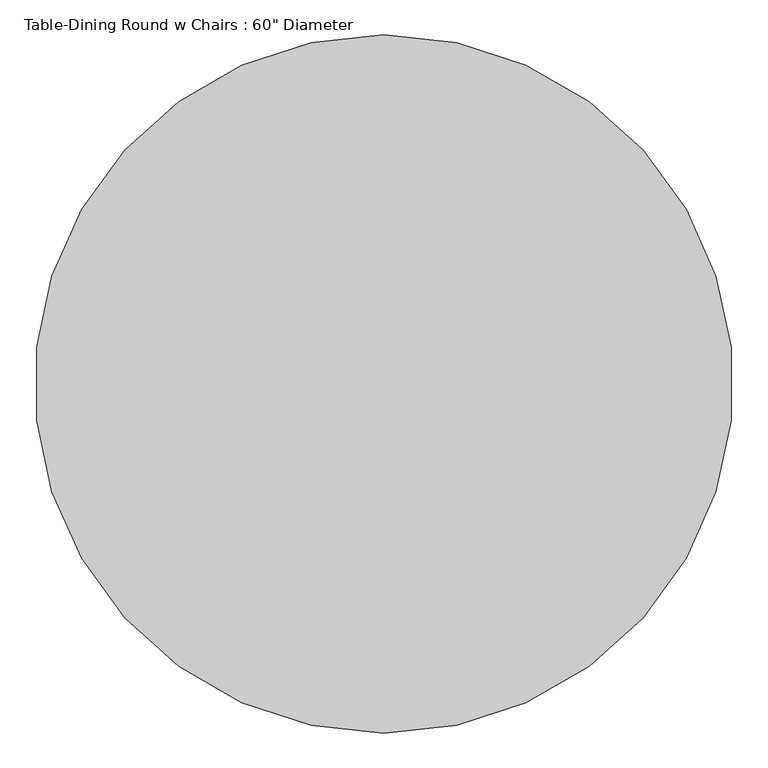
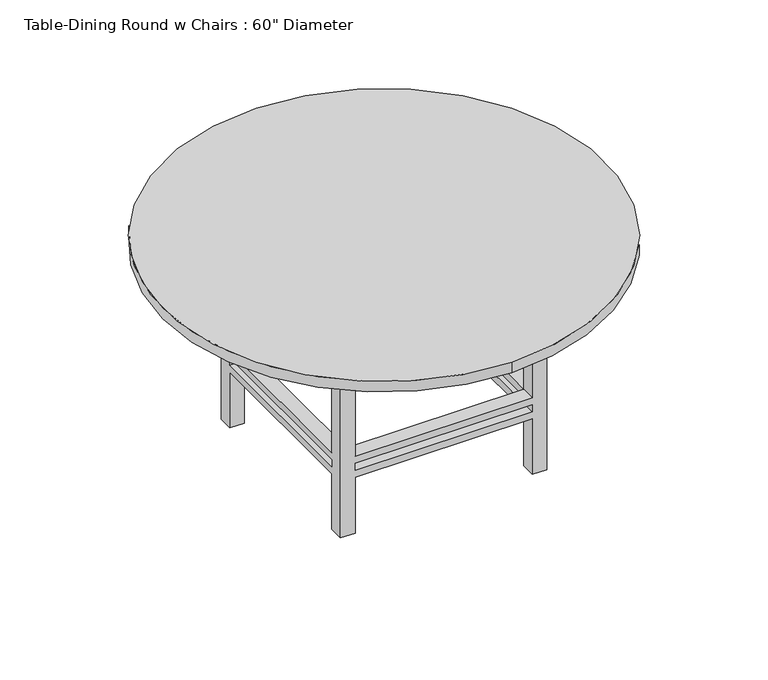
"""IFC4 building model written with IfcOpenShell, lengths in millimetres: furniture geometry."""

from ifc_helpers import new_model, si_unit, point, frame, frame_2d, origin, place, context, project, spatial, polyline, circle_curve, trimmed, segment, composite_curve, outline, extrude, faceted_brep, source, transform, mapped, element, save


def furniture_86cdcdde(model_context):
    return source(origin(), model_context, "Body", "SolidModel", [
        extrude(outline(polyline([(484.6819672, 196.1213115), (484.6819672, -565.8786885), (-277.3180328, -565.8786885), (-277.3180328, 196.1213115), (484.6819672, 196.1213115)]), holes=[polyline([(459.2819672, 170.7213115), (-251.9180328, 170.7213115), (-251.9180328, -540.4786885), (459.2819672, -540.4786885), (459.2819672, 170.7213115)])]), frame((0.0, 0.0, 647.7), z_axis=(0.0, 0.0, 1.0), x_axis=(1.0, 0.0, 0.0)), (0.0, 0.0, 1.0), 76.2),
        faceted_brep([(408.4819672, 119.9213115, 279.4), (408.4819672, -489.6786885, 279.4), (459.2819672, -489.6786885, 279.4), (459.2819672, 119.9213115, 279.4), (-201.1180328, -489.6786885, 279.4), (-201.1180328, -540.4786885, 279.4), (408.4819672, -540.4786885, 279.4), (-201.1180328, 119.9213115, 279.4), (-251.9180328, 119.9213115, 279.4), (-251.9180328, -489.6786885, 279.4), (408.4819672, 170.7213115, 279.4), (-201.1180328, 170.7213115, 279.4), (408.4819672, 119.9213115, 254.0), (-201.1180328, 119.9213115, 254.0), (-201.1180328, 170.7213115, 254.0), (408.4819672, 170.7213115, 254.0), (-201.1180328, -489.6786885, 254.0), (-251.9180328, -489.6786885, 254.0), (-251.9180328, 119.9213115, 254.0), (408.4819672, -489.6786885, 254.0), (408.4819672, -540.4786885, 254.0), (-201.1180328, -540.4786885, 254.0), (459.2819672, 119.9213115, 254.0), (459.2819672, -489.6786885, 254.0), (-251.9180328, 170.7213115, 647.7), (-201.1180328, 170.7213115, 647.7), (408.4819672, 170.7213115, 647.7), (459.2819672, 170.7213115, 647.7), (459.2819672, 170.7213115, 0.0), (408.4819672, 170.7213115, 0.0), (408.4819672, 170.7213115, 203.2), (-201.1180328, 170.7213115, 203.2), (-201.1180328, 170.7213115, 0.0), (-251.9180328, 170.7213115, 0.0), (-201.1180328, 170.7213115, 228.6), (408.4819672, 170.7213115, 228.6), (-251.9180328, 119.9213115, 647.7), (-251.9180328, 119.9213115, 0.0), (-251.9180328, 119.9213115, 203.2), (-251.9180328, -489.6786885, 203.2), (-251.9180328, -489.6786885, 0.0), (-251.9180328, -540.4786885, 0.0), (-251.9180328, -540.4786885, 647.7), (-251.9180328, -489.6786885, 647.7), (-251.9180328, -489.6786885, 228.6), (-251.9180328, 119.9213115, 228.6), (459.2819672, -540.4786885, 647.7), (408.4819672, -540.4786885, 647.7), (-201.1180328, -540.4786885, 647.7), (-201.1180328, -540.4786885, 0.0), (-201.1180328, -540.4786885, 203.2), (408.4819672, -540.4786885, 203.2), (408.4819672, -540.4786885, 0.0), (459.2819672, -540.4786885, 0.0), (408.4819672, -540.4786885, 228.6), (-201.1180328, -540.4786885, 228.6), (459.2819672, 119.9213115, 647.7), (459.2819672, -489.6786885, 647.7), (459.2819672, -489.6786885, 0.0), (459.2819672, -489.6786885, 203.2), (459.2819672, 119.9213115, 203.2), (459.2819672, 119.9213115, 0.0), (459.2819672, 119.9213115, 228.6), (459.2819672, -489.6786885, 228.6), (-201.1180328, 119.9213115, 647.7), (408.4819672, -489.6786885, 647.7), (408.4819672, 119.9213115, 647.7), (-201.1180328, -489.6786885, 647.7), (408.4819672, 119.9213115, 0.0), (-201.1180328, -489.6786885, 0.0), (-201.1180328, 119.9213115, 0.0), (408.4819672, -489.6786885, 0.0), (-201.1180328, 119.9213115, 228.6), (-201.1180328, 119.9213115, 203.2), (408.4819672, 119.9213115, 228.6), (408.4819672, 119.9213115, 203.2), (408.4819672, -489.6786885, 228.6), (408.4819672, -489.6786885, 203.2), (-201.1180328, -489.6786885, 228.6), (-201.1180328, -489.6786885, 203.2)], [[[0, 1, 2, 3]], [[1, 4, 5, 6]], [[4, 7, 8, 9]], [[7, 0, 10, 11]], [[12, 13, 14, 15]], [[13, 16, 17, 18]], [[16, 19, 20, 21]], [[19, 12, 22, 23]], [[24, 25, 11, 10, 26, 27, 28, 29, 30, 31, 32, 33], [14, 34, 35, 15]], [[36, 24, 33, 37, 38, 39, 40, 41, 42, 43, 9, 8], [17, 44, 45, 18]], [[46, 47, 6, 5, 48, 42, 41, 49, 50, 51, 52, 53], [20, 54, 55, 21]], [[28, 27, 56, 3, 2, 57, 46, 53, 58, 59, 60, 61], [22, 62, 63, 23]], [[1, 0, 12, 19]], [[4, 1, 19, 16]], [[7, 4, 16, 13]], [[0, 7, 13, 12]], [[25, 24, 36, 64]], [[47, 46, 57, 65]], [[26, 66, 56, 27]], [[48, 67, 43, 42]], [[29, 28, 61, 68]], [[49, 41, 40, 69]], [[32, 70, 37, 33]], [[52, 71, 58, 53]], [[13, 18, 45, 72]], [[64, 36, 8, 7]], [[37, 70, 73, 38]], [[14, 13, 72, 34]], [[25, 64, 7, 11]], [[70, 32, 31, 73]], [[12, 15, 35, 74]], [[66, 26, 10, 0]], [[29, 68, 75, 30]], [[22, 12, 74, 62]], [[56, 66, 0, 3]], [[68, 61, 60, 75]], [[19, 23, 63, 76]], [[65, 57, 2, 1]], [[58, 71, 77, 59]], [[20, 19, 76, 54]], [[47, 65, 1, 6]], [[71, 52, 51, 77]], [[16, 21, 55, 78]], [[67, 48, 5, 4]], [[49, 69, 79, 50]], [[17, 16, 78, 44]], [[43, 67, 4, 9]], [[69, 40, 39, 79]], [[74, 76, 63, 62]], [[76, 78, 55, 54]], [[78, 72, 45, 44]], [[72, 74, 35, 34]], [[75, 73, 31, 30]], [[73, 79, 39, 38]], [[79, 77, 51, 50]], [[77, 75, 60, 59]], [[76, 74, 75, 77]], [[78, 76, 77, 79]], [[72, 78, 79, 73]], [[74, 72, 73, 75]]]),
        extrude(outline(composite_curve([segment(trimmed(circle_curve(frame_2d((103.6819672, -184.8786885)), 762.0), [point((103.6819672, -946.8786885))], [point((103.6819672, 577.1213115))], False, "CARTESIAN"), True, "CONTINUOUS"), segment(trimmed(circle_curve(frame_2d((103.6819672, -184.8786885)), 762.0), [point((103.6819672, 577.1213115))], [point((103.6819672, -946.8786885))], False, "CARTESIAN"), True, "CONTINUOUS")], self_intersect=False)), frame((0.0, 0.0, 723.9), z_axis=(0.0, 0.0, 1.0), x_axis=(1.0, 0.0, 0.0)), (0.0, 0.0, 1.0), 38.1),
    ])


if __name__ == "__main__":
    model = new_model("IFC4")
    model_context = context("Model", 3, world=origin())
    ifc_project = project(units=[si_unit("LENGTHUNIT", "METRE", prefix="MILLI")], contexts=[model_context])
    site = spatial("IfcSite", under=ifc_project)
    building = spatial("IfcBuilding", under=site)
    placement = place(None, origin())
    furniture_shape = furniture_86cdcdde(model_context)
    element("IfcFurniture", 1, ObjectType="Table-Dining Round w Chairs : 60\" Diameter", at=placement, inside=building, context=model_context, shape_type="MappedRepresentation", body=[
        mapped(furniture_shape, transform((0.0, 0.0, 0.0), x_axis=(1.0, 0.0, 0.0), y_axis=(0.0, 1.0, 0.0), z_axis=(0.0, 0.0, 1.0))),
    ])
    save(model, "model.ifc")

# Revit data of these elements
# Type "Table-Dining Round w Chairs : 60\" Diameter"
#   Assembly Code = "E2020200"
#   Radius = 2' - 6"
#   Diameter = 5' - 0"
#   Height = 2' - 6"
#   Chairs = 6
#   Base Material = Pine
#   Top Material = Laminate, Linen, Matte
#   Default Elevation = 0
# Element 1 (IfcFurniture, "Table-Dining Round w Chairs : 60\" Diameter")
#   Materials on its faces: "Pine", "Laminate, Linen, Matte"
# Materials
#   "Pine": class "Wood", colour RGB 223 192 134, transparency 0, Description = "Pinus Echinata", Cost = 0
#   "Laminate, Linen, Matte": class "Plastic", colour RGB 249 239 230, transparency 0, Description = "Plastic Laminate - Linen, Matte", Cost = 0
